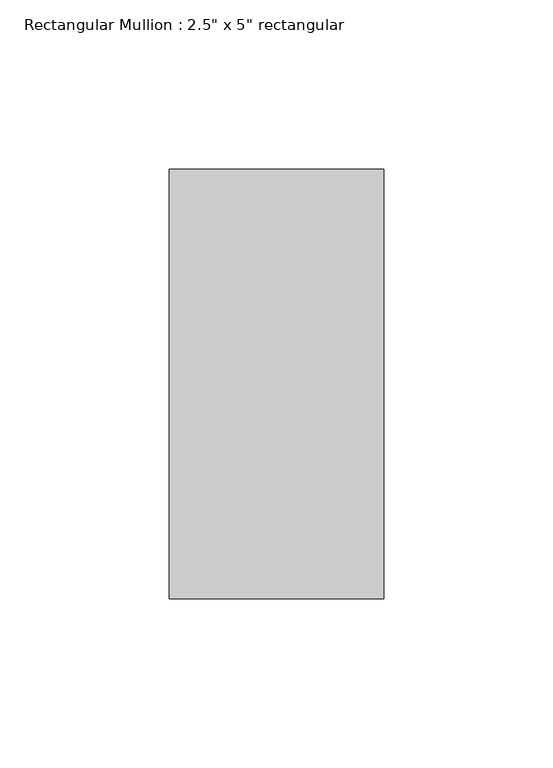
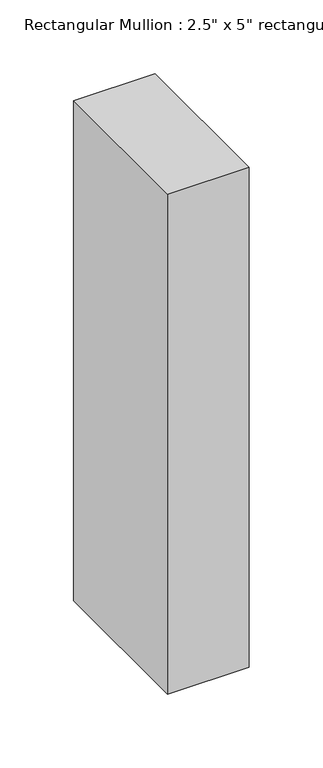
"""IFC4 building model written with IfcOpenShell, lengths in millimetres: member geometry."""

from ifc_helpers import new_model, si_unit, frame, origin, place, context, project, spatial, polyline, outline, extrude, source, transform, mapped, element, save


def member_dc106669(model_context):
    return source(origin(), model_context, "Body", "SweptSolid", [
        extrude(outline(polyline([(0.0, 63.5), (0.0, -63.5), (-63.5, -63.5), (-63.5, 63.5), (0.0, 63.5)])), frame((0.0, 0.0, -412.75), z_axis=(0.0, 0.0, 1.0), x_axis=(1.0, 0.0, 0.0)), (0.0, 0.0, 1.0), 412.75),
    ])


if __name__ == "__main__":
    model = new_model("IFC4")
    model_context = context("Model", 3, world=origin())
    ifc_project = project(units=[si_unit("LENGTHUNIT", "METRE", prefix="MILLI")], contexts=[model_context])
    site = spatial("IfcSite", under=ifc_project)
    building = spatial("IfcBuilding", under=site)
    placement = place(None, origin())
    member_shape = member_dc106669(model_context)
    element("IfcMember", 1, ObjectType="Rectangular Mullion : 2.5\" x 5\" rectangular", at=placement, inside=building, context=model_context, shape_type="MappedRepresentation", body=[
        mapped(member_shape, transform((0.0, 0.0, 0.0), x_axis=(1.0, 0.0, 0.0), y_axis=(0.0, 1.0, 0.0), z_axis=(0.0, 0.0, 1.0))),
    ])
    save(model, "model.ifc")

# Revit data of these elements
# Type "Rectangular Mullion : 2.5\" x 5\" rectangular"
#   built-in parameter 1007304 = 0.416667 (stored number, unit not read)
#   built-in parameter 1007301 = 0.104167 (stored number, unit not read)
#   built-in parameter 1007300 = 0.104167 (stored number, unit not read)
# Element 1 (IfcMember, "Rectangular Mullion : 2.5\" x 5\" rectangular")
#   Materials on its faces: "door colour"
# Materials
#   "door colour": class "Generic", colour RGB 120 120 120, transparency 0, Cost = 0
